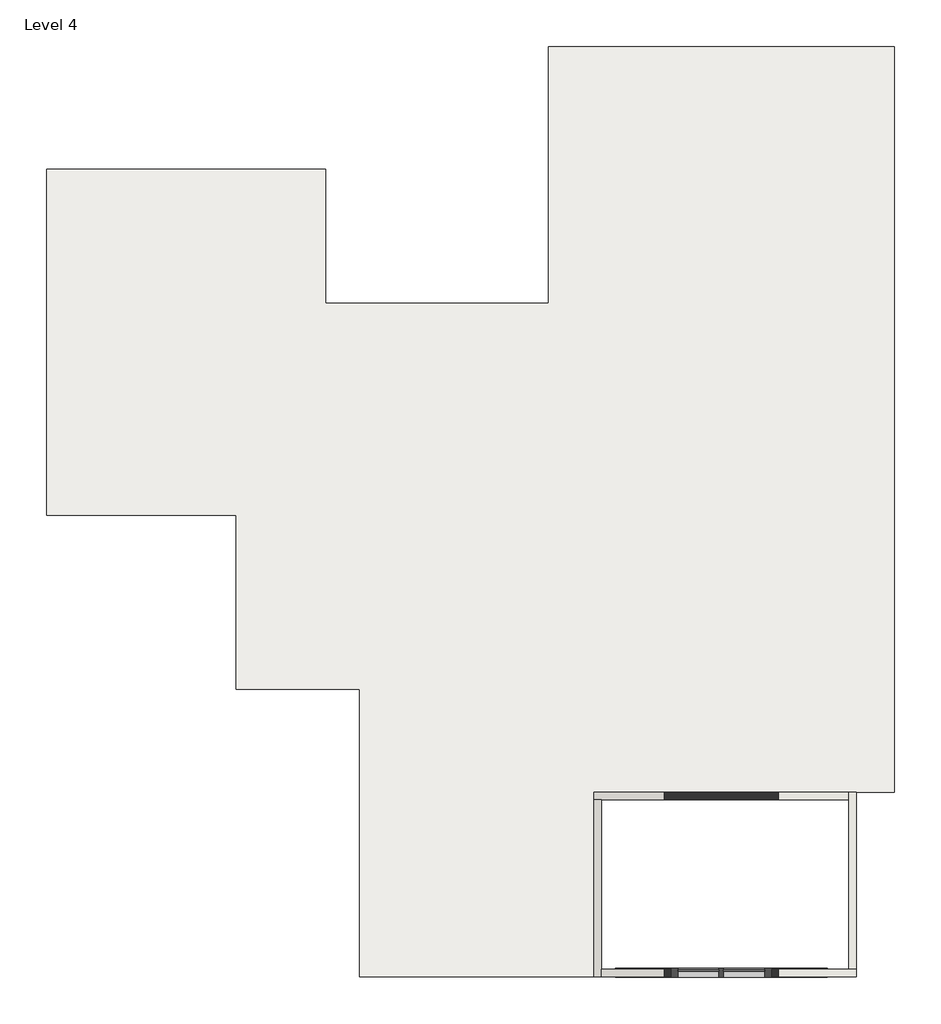
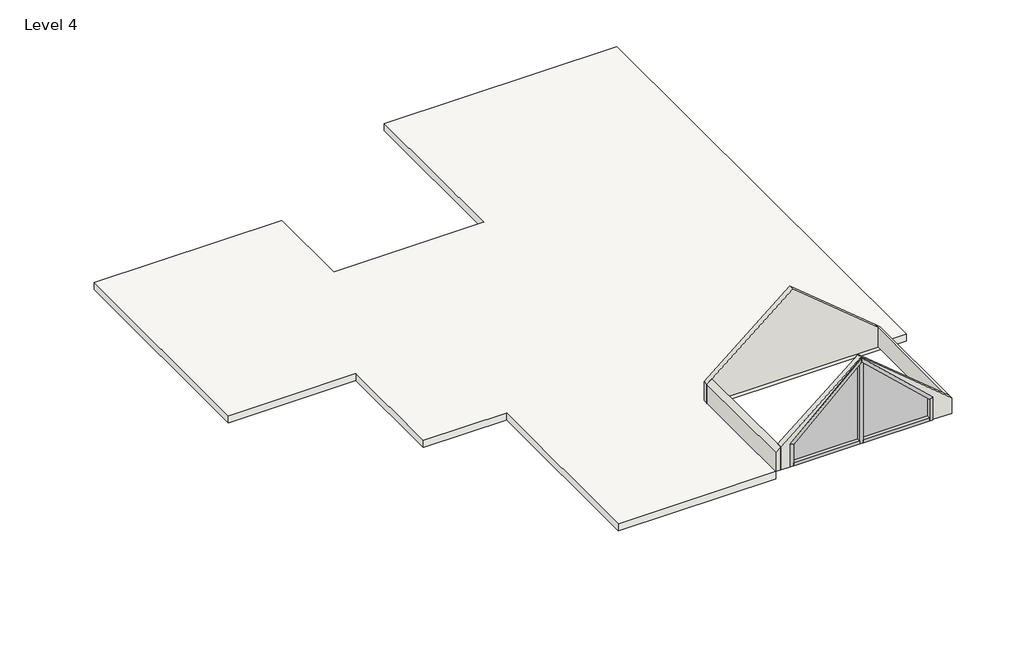
# One storey: 7 members, 4 walls, 2 plates, 1 slab.
"""IFC4 building model written with IfcOpenShell, lengths in millimetres."""

from ifc_helpers import new_model, si_unit, frame, origin, place, context, project, spatial, polyline, outline, extrude, faceted_brep, transform, mapped, element, save
from components import member_129d910c, member_d36c5697, member_cd571718, member_2e3f679f, member_5e346b9e, member_9b69c4fe, member_3f5ee701, system_panel_glazed_16cbe3df, system_panel_glazed_b4bfdf73

model = new_model("IFC4")

# Units and contexts
model_context = context("Model", 3, world=origin())
ifc_project = project(units=[si_unit("LENGTHUNIT", "METRE", prefix="MILLI")], contexts=[model_context])

# Site, building, storey
site = spatial("IfcSite", under=ifc_project)
building = spatial("IfcBuilding", under=site)
storey = spatial("IfcBuildingStorey", under=building, Name="Level 4", Elevation=6858.0)

# Members
placement = place(None, origin())
member_shape = member_129d910c(model_context)
element("IfcMember", 1, ObjectType="Rectangular Mullion : 2.5\" x 5\" rectangular", at=placement, inside=storey, context=model_context, shape_type="MappedRepresentation", body=[
    mapped(member_shape, transform((-2939.6548078, -34.5803708, 8700.27953), x_axis=(-0.6819983600624981, 0.0, 0.7313537016191708), y_axis=(0.0, -1.0, 0.0), z_axis=(0.7313537016191708, 0.0, 0.6819983600624981))),
])
member_2_shape = member_d36c5697(model_context)
element("IfcMember", 2, ObjectType="Rectangular Mullion : 2.5\" x 5\" rectangular", at=placement, inside=storey, context=model_context, shape_type="MappedRepresentation", body=[
    mapped(member_2_shape, transform((-1493.1747622, -34.5803708, 7351.4150656), x_axis=(0.6819983600625005, 0.0, 0.7313537016191687), y_axis=(0.0, -1.0, 0.0), z_axis=(0.7313537016191687, 0.0, -0.6819983600625005))),
])
member_3_shape = member_cd571718(model_context)
element("IfcMember", 3, ObjectType="Rectangular Mullion : 2.5\" x 5\" rectangular", at=placement, inside=storey, context=model_context, shape_type="MappedRepresentation", body=[
    mapped(member_3_shape, transform((-4321.6610972, -34.5803708, 6858.0), x_axis=(0.0, 0.0, -1.0), y_axis=(0.0, -1.0, 0.0), z_axis=(-1.0, 0.0, 0.0))),
])
member_4_shape = member_2e3f679f(model_context)
element("IfcMember", 4, ObjectType="Rectangular Mullion : 2.5\" x 5\" rectangular", at=placement, inside=storey, context=model_context, shape_type="MappedRepresentation", body=[
    mapped(member_4_shape, transform((-2939.6548078, -34.5803708, 6858.0), x_axis=(1.0, 0.0, 0.0), y_axis=(0.0, -1.0, 0.0), z_axis=(0.0, 0.0, -1.0))),
])
member_5_shape = member_5e346b9e(model_context)
element("IfcMember", 5, ObjectType="Rectangular Mullion : 2.5\" x 5\" rectangular", at=placement, inside=storey, context=model_context, shape_type="MappedRepresentation", body=[
    mapped(member_5_shape, transform((-2907.9048078, -34.5803708, 6858.0), x_axis=(0.0, 0.0, -1.0), y_axis=(0.0, -1.0, 0.0), z_axis=(-1.0, 0.0, 0.0))),
])
member_6_shape = member_9b69c4fe(model_context)
element("IfcMember", 6, ObjectType="Rectangular Mullion : 2.5\" x 5\" rectangular", at=placement, inside=storey, context=model_context, shape_type="MappedRepresentation", body=[
    mapped(member_6_shape, transform((-1493.1747622, -34.5803708, 6858.0), x_axis=(1.0, 0.0, 0.0), y_axis=(0.0, -1.0, 0.0), z_axis=(0.0, 0.0, -1.0))),
])
member_7_shape = member_3f5ee701(model_context)
element("IfcMember", 7, ObjectType="Rectangular Mullion : 2.5\" x 5\" rectangular", at=placement, inside=storey, context=model_context, shape_type="MappedRepresentation", body=[
    mapped(member_7_shape, transform((-4385.1610972, -34.5803708, 7352.323108), x_axis=(-1.0, 0.0, 0.0), y_axis=(0.0, -1.0, 0.0), z_axis=(0.0, 0.0, 1.0))),
])

# Plates
system_panel_glazed_shape = system_panel_glazed_16cbe3df(model_context)
element("IfcPlate", 8, ObjectType="System Panel : Glazed", at=placement, inside=storey, context=model_context, shape_type="MappedRepresentation", body=[
    mapped(system_panel_glazed_shape, transform((-3646.5329525, -34.5803708, 6921.5), x_axis=(1.0, 0.0, 0.0), y_axis=(0.0, 1.0, 0.0), z_axis=(0.0, 0.0, 1.0))),
])
system_panel_glazed_2_shape = system_panel_glazed_b4bfdf73(model_context)
element("IfcPlate", 9, ObjectType="System Panel : Glazed", at=placement, inside=storey, context=model_context, shape_type="MappedRepresentation", body=[
    mapped(system_panel_glazed_2_shape, transform((-2232.289785, -34.5803708, 6921.5), x_axis=(1.0, 0.0, 0.0), y_axis=(0.0, 1.0, 0.0), z_axis=(0.0, 0.0, 1.0))),
])

# Slab
element("IfcSlab", 10, ObjectType="6\" floor", at=placement, inside=storey, context=model_context, shape_type="SweptSolid", body=[
    extrude(outline(polyline([(-12159.3679297, 10938.2196292), (-8349.3679297, 10938.2196292), (-8349.3679297, 9109.4196292), (-5301.3679297, 9109.4196292), (-5301.3679297, 12614.6196292), (-576.9679297, 12614.6196292), (-576.9679297, 2429.2196292), (-4679.5548078, 2429.2196292), (-4679.5548078, -85.3803708), (-7879.4679297, -85.3803708), (-7879.4679297, 3838.3303652), (-9568.5679297, 3838.3303652), (-9568.5679297, 6213.8196292), (-12159.3679297, 6213.8196292), (-12159.3679297, 10938.2196292)])), frame((0.0, 0.0, 6705.6), z_axis=(0.0, 0.0, 1.0), x_axis=(1.0, 0.0, 0.0)), (0.0, 0.0, 1.0), 152.4),
])

# Walls
element("IfcWall", 11, ObjectType="4.5\" wall", at=placement, inside=storey, context=model_context, shape_type="Brep", body=[
    faceted_brep([(-1098.1548078, 16.2196292, 7187.4929406), (-1098.1548078, 16.2196292, 6858.0), (-1199.7548078, 16.2196292, 6858.0), (-1493.1747622, 16.2196292, 6858.0), (-1493.1747622, 16.2196292, 7351.4150656), (-2939.6548078, 16.2196292, 8700.27953), (-4385.1610972, 16.2196292, 7352.323108), (-4385.1610972, 16.2196292, 6858.0), (-4577.9548078, 16.2196292, 6858.0), (-4577.9548078, 16.2196292, 7355.2135756), (-2939.6548078, 16.2196292, 8707.4611946), (-1199.7548078, 16.2196292, 7271.3532581), (-1098.1548078, -85.3803708, 6858.0), (-1098.1548078, -85.3803708, 7187.4929406), (-2939.6548078, -85.3803708, 8707.4611946), (-4577.9548078, -85.3803708, 7355.2135756), (-4577.9548078, -85.3803708, 6858.0), (-4385.1610972, -85.3803708, 6858.0), (-4385.1610972, -85.3803708, 7352.323108), (-2939.6548078, -85.3803708, 8700.27953), (-1493.1747622, -85.3803708, 7351.4150656), (-1493.1747622, -85.3803708, 6858.0)], [[[0, 1, 2, 3, 4, 5, 6, 7, 8, 9, 10, 11]], [[12, 13, 14, 15, 16, 17, 18, 19, 20, 21]], [[1, 12, 21, 3, 2]], [[16, 8, 7, 17]], [[1, 0, 13, 12]], [[9, 8, 16, 15]], [[18, 6, 5, 19]], [[19, 5, 4, 20]], [[20, 4, 3, 21]], [[6, 18, 17, 7]], [[13, 0, 11, 10, 14]], [[9, 15, 14, 10]]]),
])
element("IfcWall", 12, ObjectType="4.5\" wall", at=placement, inside=storey, context=model_context, shape_type="Brep", body=[
    faceted_brep([(-1199.7548078, 2429.2196292, 6858.0), (-1199.7548078, 2327.6196292, 6858.0), (-1199.7548078, 16.2196292, 6858.0), (-1199.7548078, 16.2196292, 7271.3532581), (-1199.7548078, 2327.6196292, 7271.3532581), (-1199.7548078, 2429.2196292, 7271.3532581), (-1098.1548078, 2429.2196292, 6858.0), (-1098.1548078, 2429.2196292, 7187.4929406), (-1098.1548078, 16.2196292, 7187.4929406), (-1098.1548078, 16.2196292, 6858.0)], [[[0, 1, 2, 3, 4, 5]], [[6, 7, 8, 9]], [[2, 1, 0, 6, 9]], [[0, 5, 7, 6]], [[3, 2, 9, 8]], [[5, 4, 3, 8, 7]]]),
])
element("IfcWall", 13, ObjectType="4.5\" wall", at=placement, inside=storey, context=model_context, shape_type="Brep", body=[
    faceted_brep([(-4679.5548078, 2327.6196292, 6858.0), (-4577.9548078, 2327.6196292, 6858.0), (-1199.7548078, 2327.6196292, 6858.0), (-1199.7548078, 2327.6196292, 7271.3532581), (-2939.6548078, 2327.6196292, 8707.4611946), (-4577.9548078, 2327.6196292, 7355.2135756), (-4679.5548078, 2327.6196292, 7271.3532581), (-4679.5548078, 2429.2196292, 6858.0), (-4679.5548078, 2429.2196292, 7271.3532581), (-2939.6548078, 2429.2196292, 8707.4611946), (-1199.7548078, 2429.2196292, 7271.3532581), (-1199.7548078, 2429.2196292, 6858.0)], [[[0, 1, 2, 3, 4, 5, 6]], [[7, 8, 9, 10, 11]], [[2, 1, 0, 7, 11]], [[0, 6, 8, 7]], [[3, 2, 11, 10]], [[6, 5, 4, 9, 8]], [[4, 3, 10, 9]]]),
])
element("IfcWall", 14, ObjectType="4.5\" wall", at=placement, inside=storey, context=model_context, shape_type="Brep", body=[
    faceted_brep([(-4577.9548078, -85.3803708, 6858.0), (-4577.9548078, 16.2196292, 6858.0), (-4577.9548078, 2327.6196292, 6858.0), (-4577.9548078, 2327.6196292, 7355.2135756), (-4577.9548078, 16.2196292, 7355.2135756), (-4577.9548078, -85.3803708, 7355.2135756), (-4679.5548078, -85.3803708, 6858.0), (-4679.5548078, -85.3803708, 7271.3532581), (-4679.5548078, 2327.6196292, 7271.3532581), (-4679.5548078, 2327.6196292, 6858.0)], [[[0, 1, 2, 3, 4, 5]], [[6, 7, 8, 9]], [[2, 1, 0, 6, 9]], [[0, 5, 7, 6]], [[3, 2, 9, 8]], [[5, 4, 3, 8, 7]]]),
])

save(model, "model.ifc")

# Revit data of these elements
# Type "Rectangular Mullion : 2.5\" x 5\" rectangular"
#   built-in parameter 1007304 = 0.416667 (stored number, unit not read)
#   built-in parameter 1007301 = 0.104167 (stored number, unit not read)
#   built-in parameter 1007300 = 0.104167 (stored number, unit not read)
# Type "System Panel : Glazed"
#   Construction Type Id = "GSP4R"
#   Analytic Construction = "1/8 in Pilkington single glazing"
#   Visual Light Transmittance = 0.9
#   Solar Heat Gain Coefficient = 0.86
#   Heat Transfer Coefficient (U) = 1.18115 BTU/(h·ft²·°F)
#   Define Thermal Properties by = 1
# Type "6\" floor"
#   Assembly Code = "B1010"
#   Function = 0
#   Layers, outside or top first: 0' - 6" "Laminate, Ivory, Matte" (function 1)
# Type "4.5\" wall"
#   Assembly Code = "B2010"
#   Layers, outside or top first: 0' - 4" "Laminate, Ivory, Matte" (function 1)
# Elements 1, 2, 3, 4, 5, 6, 7 (IfcMember, "Rectangular Mullion : 2.5\" x 5\" rectangular")
#   Phase Created = New Construction
#   Materials on its faces: "door colour"
# Elements 8, 9 (IfcPlate, "System Panel : Glazed")
#   Phase Created = New Construction
#   Materials on its faces: "Glass"
# Element 10 (IfcSlab, "6\" floor")
#   built-in parameter 1001955 = 3.14159 (stored number, unit not read)
#   Height Offset From Level = 0' - 0"
#   Phase Created = New Construction
#   Materials on its faces: "Laminate, Ivory, Matte"
# Elements 11, 12, 13, 14 (IfcWall, "4.5\" wall")
#   Top Offset = 2' - 0"
#   Base Offset = 0' - 0"
#   wall height = 2' - 6"
#   Phase Created = New Construction
#   Base Constraint = Level 4
#   Top Constraint = Level 5
#   Materials on its faces: "Laminate, Ivory, Matte"
# Materials
#   "Laminate, Ivory, Matte": class "Plastic", colour RGB 247 247 239, transparency 0, Description = "Plastic Laminate - Ivory, Matte", Cost = 0
#   "door colour": class "Generic", colour RGB 120 120 120, transparency 0, Cost = 0
#   "Glass": class "Glass", colour RGB 0 128 192, transparency 0.75, Description = "Soda Lime Glass", Cost = 0
